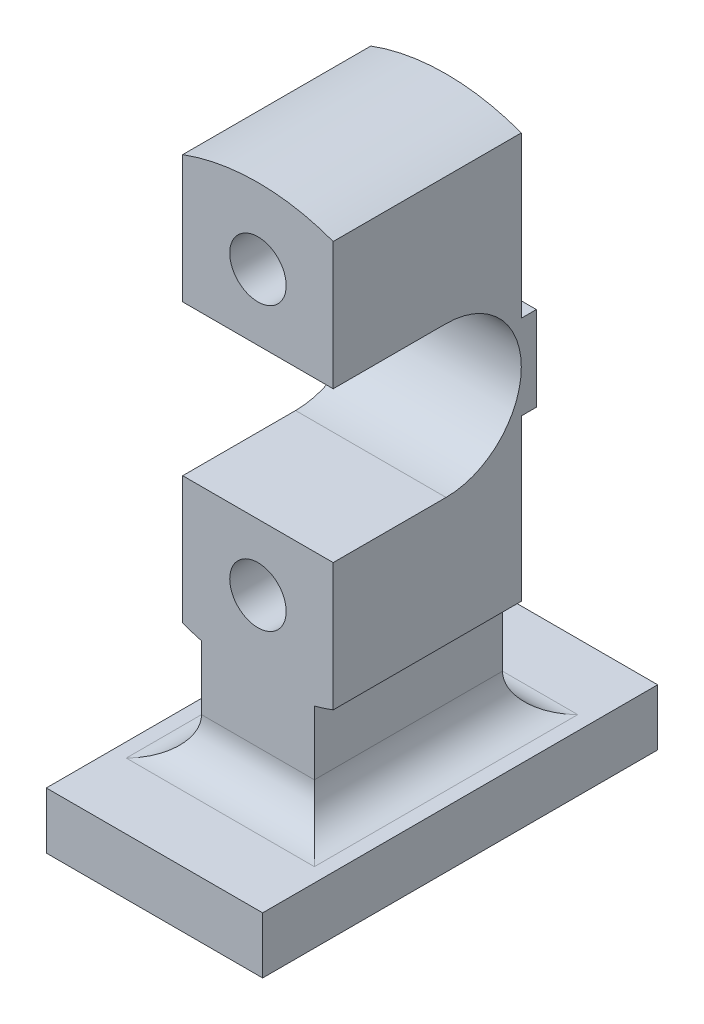
SolidWorks part; units mm, degrees
material "Plain Carbon Steel"
ref_plane "Front Plane" through (0, 0, 0) normal (0, 0, 1) x (1, 0, 0)
ref_plane "Top Plane" through (0, 0, 0) normal (0, 1, 0) x (1, 0, 0)
ref_plane "Right Plane" through (0, 0, 0) normal (1, 0, 0) x (0, 0, -1)
sketch "Upright Profile Sketch" plane through (0, 0, 0) normal (0, 0, 1) x (1, 0, 0)
  line L0 (0, 0) -> (-179.2608, 0) construction
  line L2 (-40, -107.8193) -> (-40, 107.8193)
  line L4 (40, -107.8193) -> (40, 107.8193)
  line L5 (-40, -107.8193) -> (40, 107.8193) construction
  line L6 (-40, 107.8193) -> (40, -107.8193) construction
  line L7 (-30, -165) -> (30, -165)
  line L9 (-30, -111.018) -> (-30, -165)
  line L11 (30, -111.018) -> (30, -165)
  line L16 (0, 0) -> (0, -236.4659) construction
  line L17 (-89.7025, -195) -> (102.7303, -195) construction
  arc A0 (-40, 107.8193) -> (40, 107.8193) centre (0, 0) cw
  arc A1 (-40, -107.8193) -> (-30, -111.018) centre (0, 0) ccw
  circle A2 centre (0, 75) radius 15
  circle A3 centre (0, -75) radius 15
  arc A4 (30, -111.018) -> (40, -107.8193) centre (0, 0) ccw
  point P0 (0, 0)
  point P12 (0, 115)
  dimension "D1" = 115
  dimension "D8" = 75
  dimension "30" = 30
  dimension "D2" = 60
  dimension "D3" = 30
  dimension "D4" = 195
  dimension "D5" = 80
  dimension "D6" = 30
  dimension "D7" = 310
extrude "Upright Body" add sketch "Upright Profile Sketch" along normal mid plane 100
sketch "Base Plate Sketch" plane through (0, -165, 0) normal (0, -1, 0) x (1, 0, 0)
  line L1 (-57.5, -105) -> (57.5, -105)
  line L2 (-57.5, -105) -> (-57.5, 105)
  line L3 (-57.5, 105) -> (57.5, 105)
  line L4 (57.5, -105) -> (57.5, 105)
  line L5 (-57.5, -105) -> (57.5, 105) construction
  line L6 (-57.5, 105) -> (57.5, -105) construction
  point P0 (0, 0)
  dimension "D1" = 210
  dimension "D2" = 115
extrude "Base Plate 210x115x30" add sketch "Base Plate Sketch" along normal blind 30
fillet "Base Blend Fillet R20" radius 20 4 edges at (0, -165, -50) (-30, -165, 0) (0, -165, 50) (30, -165, 0)
sketch "Side Boss Sketch" plane through (40, 0, 0) normal (1, 0, 0) x (0, 0, -1)
  line L0 (50, -107.8193) -> (50, 107.8193) construction
  line L1 (50, 22.5) -> (58, 22.5)
  line L2 (50, 22.5) -> (50, -22.5)
  line L3 (50, -22.5) -> (58, -22.5)
  line L4 (58, 22.5) -> (58, -22.5)
  point P6 (50, 0)
  dimension "D1" = 8
  dimension "D2" = 22.5
extrude "Side Boss" add sketch "Side Boss Sketch" against normal up to surface (80 mm away) up to face at (-40, 0, 0)
sketch "Upright Cut Sketch" plane through (40, 0, 0) normal (1, 0, 0) x (0, 0, -1)
  line L0 (10, 40) -> (-50, 40)
  line L1 (-50, -107.8193) -> (-50, 107.8193) construction
  line L2 (10, -40) -> (-50, -40)
  line L3 (-50, -40) -> (-50, 40)
  line L4 (10, 40) -> (10, -40) construction
  arc A0 (10, -40) -> (10, 40) centre (10, 0) ccw
  dimension "D1" = 80
  dimension "D2" = 60
extrude "Upright Profile Cut" cut sketch "Upright Cut Sketch" against normal up to surface (80 mm away) up to face at (-40, 0, -27)
